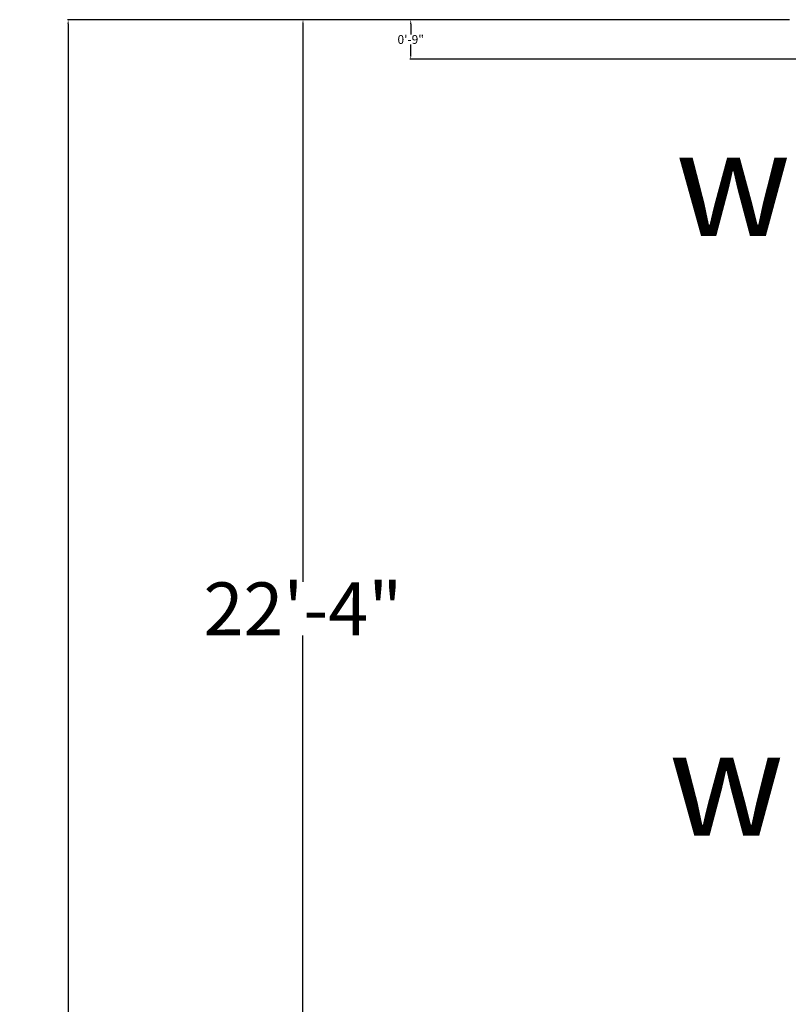
# Model space of a CAD drawing. Units: inches. Extents: x 409 to 7572, y 7 to 725.
# Tile 10 of 38: x 1521 to 1696, y 449 to 673. Entities that reach past the tile are written whole.
import ezdxf

# ---------------------------------------------------------------- set-up
doc = ezdxf.new("R2010")
doc.units = ezdxf.units.IN
doc.header["$MEASUREMENT"] = 0
doc.layers.add('A-ANNO-DIMS', color=2, linetype='Continuous', lineweight=18)
doc.layers.add('A-ANNO-SYMB', color=3, linetype='Continuous', lineweight=25)
doc.styles.get("Standard").update_dxf_attribs({"font": 'arial.ttf'})
doc.dimstyles.get("Standard").update_dxf_attribs({"dimtxt": 2, "dimasz": 1, "dimexe": 0.18, "dimexo": 0.0625, "dimgap": 0.09, "dimtad": 0, "dimtih": 1, "dimtoh": 1, "dimdec": 0, "dimzin": 0, "dimdsep": 46, "dimlunit": 3, "dimtxsty": 'Standard', "dimcen": 0.09, "dimadec": 0, "dimazin": 0, "dimtfac": 1, "dimtdec": 0, "dimtofl": 0, "dimtmove": 0, "dimatfit": 3, "dimfxl": 1, "dimtolj": 1, "dimtzin": 0, "dimarcsym": 0})

# ---------------------------------------------------------------- blocks, each defined once
blk = doc.blocks.new('*D48')
at = {"layer": 'A-ANNO-DIMS', "color": 0, "lineweight": -2, "transparency": 16777216}
for p, q in [((1696.26, 672.53), (1585.36, 672.53)), ((1585.54, 671.53), (1585.54, 544.65)), ((1585.54, 405.53), (1585.54, 532.42)), ((1696.26, 404.53), (1585.36, 404.53))]:
    blk.add_line(p, q, dxfattribs=at)
at = {"layer": 'A-ANNO-DIMS', "color": 0, "transparency": 16777216}
for points in [[(1585.37, 671.53), (1585.71, 671.53), (1585.54, 672.53)], [(1585.37, 405.53), (1585.71, 405.53), (1585.54, 404.53)]]:
    blk.add_solid(points, dxfattribs=at)
at = {"layer": 'DEFPOINTS', "color": 0, "transparency": 16777216}
for p in [(1696.32, 672.53), (1585.54, 404.53), (1696.32, 404.53)]:
    blk.add_point(p, dxfattribs=at)
at = {"layer": 'A-ANNO-DIMS', "color": 0, "transparency": 16777216, "insert": (1585.54, 538.53), "char_height": 2, "attachment_point": 5}
blk.add_mtext('\\A1;{\\H6x;22\'-4"}', dxfattribs=at)
blk = doc.blocks.new('*D37')
at = {"layer": 'A-ANNO-DIMS', "color": 0, "lineweight": -2, "transparency": 16777216}
for p, q in [((1696.26, 672.53), (1531.9, 672.53)), ((1532.08, 671.53), (1532.08, 420.75)), ((1532.08, 157.53), (1532.08, 408.31)), ((1696.26, 156.53), (1531.9, 156.53))]:
    blk.add_line(p, q, dxfattribs=at)
at = {"layer": 'A-ANNO-DIMS', "color": 0, "transparency": 16777216}
for points in [[(1531.91, 671.53), (1532.25, 671.53), (1532.08, 672.53)], [(1531.91, 157.53), (1532.25, 157.53), (1532.08, 156.53)]]:
    blk.add_solid(points, dxfattribs=at)
at = {"layer": 'DEFPOINTS', "color": 0, "transparency": 16777216}
for p in [(1696.32, 672.53), (1532.08, 156.53), (1696.32, 156.53)]:
    blk.add_point(p, dxfattribs=at)
at = {"layer": 'A-ANNO-DIMS', "color": 0, "transparency": 16777216, "insert": (1532.08, 414.53), "char_height": 2, "attachment_point": 5}
blk.add_mtext("\\A1;{\\H6x;43'}", dxfattribs=at)
blk = doc.blocks.new('*D178')
at = {"layer": 'A-ANNO-DIMS', "color": 0, "lineweight": -2, "transparency": 16777216}
for p, q in [((1696.26, 672.53), (1609.89, 672.53)), ((1610.07, 671.53), (1610.07, 669.14)), ((1610.07, 664.53), (1610.07, 666.92)), ((1705.26, 663.53), (1609.89, 663.53))]:
    blk.add_line(p, q, dxfattribs=at)
at = {"layer": 'A-ANNO-DIMS', "color": 0, "transparency": 16777216}
for points in [[(1609.9, 671.53), (1610.24, 671.53), (1610.07, 672.53)], [(1609.9, 664.53), (1610.24, 664.53), (1610.07, 663.53)]]:
    blk.add_solid(points, dxfattribs=at)
at = {"layer": 'DEFPOINTS', "color": 0, "transparency": 16777216}
for p in [(1696.32, 672.53), (1610.07, 663.53), (1705.32, 663.53)]:
    blk.add_point(p, dxfattribs=at)
at = {"layer": 'A-ANNO-DIMS', "color": 0, "transparency": 16777216, "insert": (1610.07, 668.03), "char_height": 2, "attachment_point": 5}
blk.add_mtext('\\A1;0\'-9"', dxfattribs=at)

msp = doc.modelspace()

# ---------------------------------------------------------------- texts
at = {"layer": 'A-ANNO-SYMB', "char_height": 24, "attachment_point": 1}
for insert in [(1670.33, 647.34), (1668.8, 510.91)]:
    msp.add_mtext_dynamic_manual_height_columns('w', width=18.2582, gutter_width=1, heights=[0], dxfattribs=dict(at, insert=insert))

# ---------------------------------------------------------------- dimensions: what is measured, and where the dimension line sits
at = {"layer": 'A-ANNO-DIMS'}
for base, p2, picture, middle in [((1532.08, 156.53), (1696.32, 156.53), '*D37', (1532.08, 414.53)), ((1585.54, 404.53), (1696.32, 404.53), '*D48', (1585.54, 538.53))]:
    dim = msp.add_linear_dim(base=base, p1=(1696.32, 672.53), p2=p2, angle=90, text='{\\H6x;<>}', dimstyle='Standard', override={"dimclrd": 0, "dimclre": 0, "dimclrt": 0}, dxfattribs=at)
    dim.commit()
    dim.dimension.update_dxf_attribs({"geometry": picture, "text_midpoint": middle})
dim = msp.add_linear_dim(base=(1610.07, 663.53), p1=(1696.32, 672.53), p2=(1705.32, 663.53), angle=90, dimstyle='Standard', override={"dimdec": 1, "dimlfac": 1, "dimrnd": 0, "dimzin": 1, "dimdsep": 46, "dimlunit": 4, "dimfrac": 2}, dxfattribs=at)
dim.commit()
dim.dimension.update_dxf_attribs({"geometry": '*D178', "text_midpoint": (1610.07, 668.03)})

doc.saveas('drawing.dxf')
